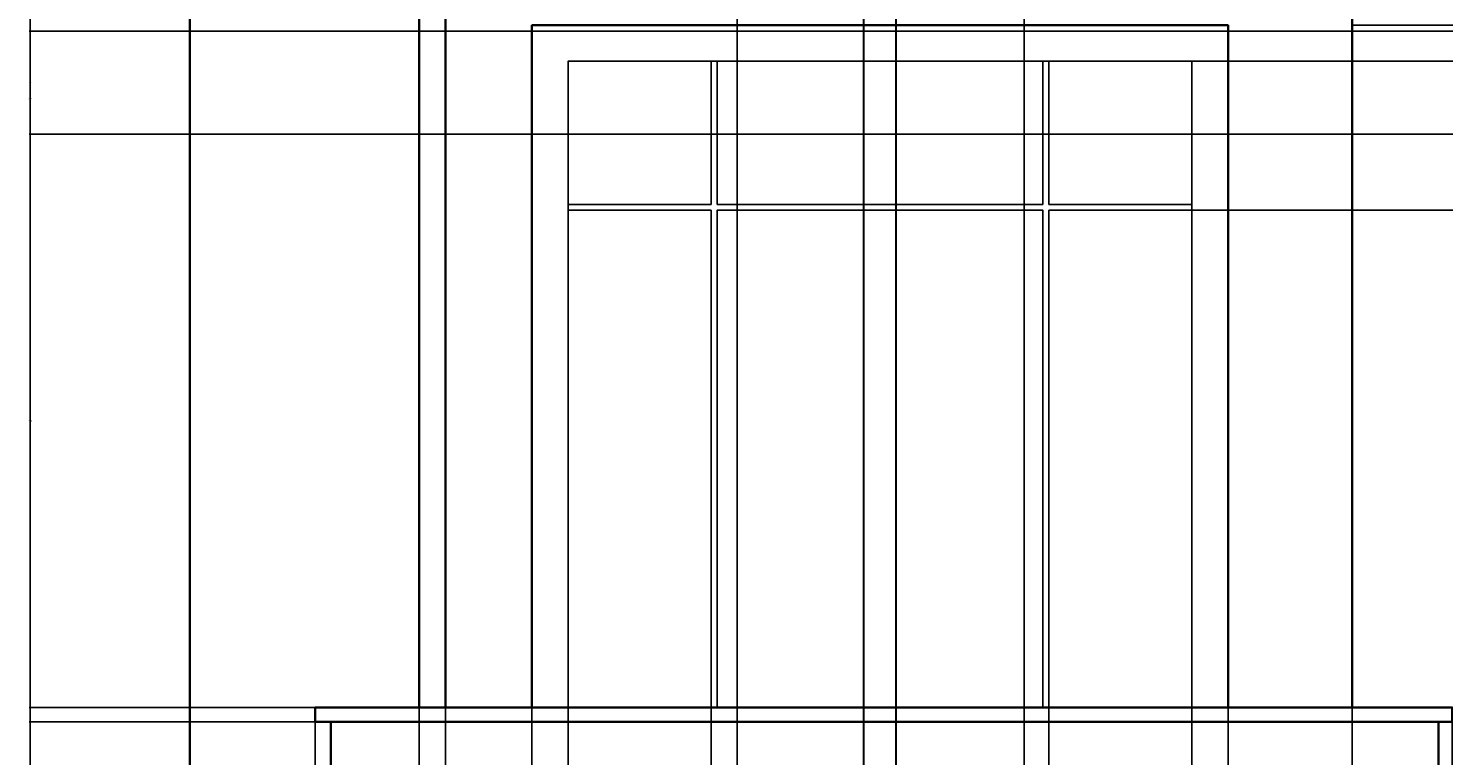
# Model space of a CAD drawing. Units: feet. Extents: x 4092 to 5585, y 725 to 1390.
# Tile 4 of 7: x 4921 to 5204, y 1001 to 1146. Entities that reach past the tile are written whole.
import ezdxf

# ---------------------------------------------------------------- set-up
doc = ezdxf.new("R2010")
doc.units = ezdxf.units.FT
for name, color, linetype, lineweight in [('A-ANNO-DIMS', 2, 'Continuous', 18), ('A-ELEV', 7, 'Continuous', 35), ('A-GLAZ', 4, 'Continuous', 25)]:
    doc.layers.add(name, color=color, linetype=linetype, lineweight=lineweight)
doc.styles.get("Standard").update_dxf_attribs({"font": 'arial.ttf'})
doc.dimstyles.get("Standard").update_dxf_attribs({"dimtxt": 0.18, "dimasz": 0.18, "dimexe": 0.18, "dimexo": 0.0625, "dimgap": 0.09, "dimtad": 0, "dimtih": 1, "dimtoh": 1, "dimdec": 1, "dimzin": 0, "dimdsep": 46, "dimlunit": 3, "dimtxsty": 'Standard', "dimcen": 0.09, "dimadec": 0, "dimazin": 0, "dimtfac": 1, "dimtdec": 1, "dimtofl": 0, "dimtmove": 0, "dimatfit": 3, "dimfxl": 1, "dimtolj": 1, "dimtzin": 0, "dimarcsym": 0})

# ---------------------------------------------------------------- blocks, each defined once
blk = doc.blocks.new('*D18')
at = {"layer": 'A-ANNO-DIMS', "color": 0, "lineweight": -2, "transparency": 16777216}
for p, q in [((4978.29, 1010.79), (4921.27, 1010.79)), ((4921.45, 1010.61), (4921.45, 981.18)), ((4921.45, 951.38), (4921.45, 980.81)), ((5021.54, 951.2), (4921.27, 951.2))]:
    blk.add_line(p, q, dxfattribs=at)
at = {"layer": 'A-ANNO-DIMS', "color": 0, "transparency": 16777216}
for points in [[(4921.42, 1010.61), (4921.48, 1010.61), (4921.45, 1010.79)], [(4921.42, 951.38), (4921.48, 951.38), (4921.45, 951.2)]]:
    blk.add_solid(points, dxfattribs=at)
at = {"layer": 'Defpoints', "color": 0, "transparency": 16777216}
for p in [(4921.45, 1010.79), (4978.36, 1010.79), (5021.61, 951.2)]:
    blk.add_point(p, dxfattribs=at)
at = {"layer": 'A-ANNO-DIMS', "color": 0, "transparency": 16777216, "insert": (4921.45, 981), "char_height": 0.18, "attachment_point": 5}
blk.add_mtext('\\A1;59.59', dxfattribs=at)
blk = doc.blocks.new('*D19')
at = {"layer": 'A-ANNO-DIMS', "color": 0, "lineweight": -2, "transparency": 16777216}
for p, q in [((4953.23, 1253.95), (4921.27, 1253.95)), ((4921.45, 1253.77), (4921.45, 1132.55)), ((4921.45, 1010.97), (4921.45, 1132.19)), ((4978.29, 1010.79), (4921.27, 1010.79))]:
    blk.add_line(p, q, dxfattribs=at)
at = {"layer": 'A-ANNO-DIMS', "color": 0, "transparency": 16777216}
for points in [[(4921.42, 1253.77), (4921.48, 1253.77), (4921.45, 1253.95)], [(4921.42, 1010.97), (4921.48, 1010.97), (4921.45, 1010.79)]]:
    blk.add_solid(points, dxfattribs=at)
at = {"layer": 'Defpoints', "color": 0, "transparency": 16777216}
for p in [(4921.45, 1253.95), (4953.29, 1253.95), (4978.36, 1010.79)]:
    blk.add_point(p, dxfattribs=at)
at = {"layer": 'A-ANNO-DIMS', "color": 0, "transparency": 16777216, "insert": (4921.45, 1132.37), "char_height": 0.18, "attachment_point": 5}
blk.add_mtext('\\A1;243.16', dxfattribs=at)
blk = doc.blocks.new('*D39')
at = {"layer": 'A-ANNO-DIMS', "color": 0, "lineweight": -2, "transparency": 16777216}
for p, q in [((5087.84, 808.72), (5087.84, 1389.85)), ((5088.02, 1389.67), (5090.69, 1389.67)), ((5094.12, 1389.67), (5091.45, 1389.67)), ((5094.3, 808.72), (5094.3, 1389.85))]:
    blk.add_line(p, q, dxfattribs=at)
at = {"layer": 'A-ANNO-DIMS', "color": 0, "transparency": 16777216}
for points in [[(5088.02, 1389.7), (5088.02, 1389.64), (5087.84, 1389.67)], [(5094.12, 1389.7), (5094.12, 1389.64), (5094.3, 1389.67)]]:
    blk.add_solid(points, dxfattribs=at)
at = {"layer": 'Defpoints', "color": 0, "transparency": 16777216}
for p in [(5094.3, 1389.67), (5087.84, 808.65), (5094.3, 808.65)]:
    blk.add_point(p, dxfattribs=at)
at = {"layer": 'A-ANNO-DIMS', "color": 0, "transparency": 16777216, "insert": (5091.07, 1389.67), "char_height": 0.18, "attachment_point": 5}
blk.add_mtext('\\A1;6.461', dxfattribs=at)
blk = doc.blocks.new('*D40')
at = {"layer": 'A-ANNO-DIMS', "color": 0, "lineweight": -2, "transparency": 16777216}
for p, q in [((5062.58, 907.22), (5062.58, 1389.85)), ((5062.76, 1389.67), (5074.7, 1389.67)), ((5087.57, 1389.67), (5075.63, 1389.67)), ((5087.75, 907.22), (5087.75, 1389.85))]:
    blk.add_line(p, q, dxfattribs=at)
at = {"layer": 'A-ANNO-DIMS', "color": 0, "transparency": 16777216}
for points in [[(5062.76, 1389.7), (5062.76, 1389.64), (5062.58, 1389.67)], [(5087.57, 1389.7), (5087.57, 1389.64), (5087.75, 1389.67)]]:
    blk.add_solid(points, dxfattribs=at)
at = {"layer": 'Defpoints', "color": 0, "transparency": 16777216}
for p in [(5087.75, 1389.67), (5062.58, 907.16), (5087.75, 907.16)]:
    blk.add_point(p, dxfattribs=at)
at = {"layer": 'A-ANNO-DIMS', "color": 0, "transparency": 16777216, "insert": (5075.16, 1389.67), "char_height": 0.18, "attachment_point": 5}
blk.add_mtext('\\A1;25.164', dxfattribs=at)
blk = doc.blocks.new('*D41')
at = {"layer": 'A-ANNO-DIMS', "color": 0, "lineweight": -2, "transparency": 16777216}
for p, q in [((5087.75, 907.22), (5087.75, 1389.85)), ((5087.93, 1389.67), (5090.59, 1389.67)), ((5094.04, 1389.67), (5091.38, 1389.67)), ((5094.22, 907.22), (5094.22, 1389.85))]:
    blk.add_line(p, q, dxfattribs=at)
at = {"layer": 'A-ANNO-DIMS', "color": 0, "transparency": 16777216}
for points in [[(5087.93, 1389.7), (5087.93, 1389.64), (5087.75, 1389.67)], [(5094.04, 1389.7), (5094.04, 1389.64), (5094.22, 1389.67)]]:
    blk.add_solid(points, dxfattribs=at)
at = {"layer": 'Defpoints', "color": 0, "transparency": 16777216}
for p in [(5094.22, 1389.67), (5087.75, 907.16), (5094.22, 907.16)]:
    blk.add_point(p, dxfattribs=at)
at = {"layer": 'A-ANNO-DIMS', "color": 0, "transparency": 16777216, "insert": (5090.98, 1389.67), "char_height": 0.18, "attachment_point": 5}
blk.add_mtext('\\A1;6.474', dxfattribs=at)
blk = doc.blocks.new('*D42')
at = {"layer": 'A-ANNO-DIMS', "color": 0, "lineweight": -2, "transparency": 16777216}
for p, q in [((5094.22, 907.22), (5094.22, 1389.85)), ((5094.4, 1389.67), (5106.69, 1389.67)), ((5119.64, 1389.67), (5107.34, 1389.67)), ((5119.82, 907.22), (5119.82, 1389.85))]:
    blk.add_line(p, q, dxfattribs=at)
at = {"layer": 'A-ANNO-DIMS', "color": 0, "transparency": 16777216}
for points in [[(5094.4, 1389.7), (5094.4, 1389.64), (5094.22, 1389.67)], [(5119.64, 1389.7), (5119.64, 1389.64), (5119.82, 1389.67)]]:
    blk.add_solid(points, dxfattribs=at)
at = {"layer": 'Defpoints', "color": 0, "transparency": 16777216}
for p in [(5119.82, 1389.67), (5094.22, 907.16), (5119.82, 907.16)]:
    blk.add_point(p, dxfattribs=at)
at = {"layer": 'A-ANNO-DIMS', "color": 0, "transparency": 16777216, "insert": (5107.02, 1389.67), "char_height": 0.18, "attachment_point": 5}
blk.add_mtext('\\A1;25.6', dxfattribs=at)
blk = doc.blocks.new('*D46')
at = {"layer": 'A-ANNO-DIMS', "color": 0, "lineweight": -2, "transparency": 16777216}
for p, q in [((4978.29, 1007.95), (4921.27, 1007.95)), ((4921.45, 1007.77), (4921.45, 986.89)), ((4921.45, 965.66), (4921.45, 986.53)), ((4981.38, 965.48), (4921.27, 965.48))]:
    blk.add_line(p, q, dxfattribs=at)
at = {"layer": 'A-ANNO-DIMS', "color": 0, "transparency": 16777216}
for points in [[(4921.42, 1007.77), (4921.48, 1007.77), (4921.45, 1007.95)], [(4921.42, 965.66), (4921.48, 965.66), (4921.45, 965.48)]]:
    blk.add_solid(points, dxfattribs=at)
at = {"layer": 'Defpoints', "color": 0, "transparency": 16777216}
for p in [(4921.45, 1007.95), (4978.36, 1007.95), (4981.44, 965.48)]:
    blk.add_point(p, dxfattribs=at)
at = {"layer": 'A-ANNO-DIMS', "color": 0, "transparency": 16777216, "insert": (4921.45, 986.71), "char_height": 0.18, "attachment_point": 5}
blk.add_mtext('\\A1;42.47', dxfattribs=at)
blk = doc.blocks.new('*D47')
at = {"layer": 'A-ANNO-DIMS', "color": 0, "lineweight": -2, "transparency": 16777216}
for p, q in [((4978.36, 1010.73), (4978.36, 725.07)), ((4999.11, 1010.73), (4999.11, 725.07)), ((4978.54, 725.25), (4988.34, 725.25)), ((4998.93, 725.25), (4989.13, 725.25))]:
    blk.add_line(p, q, dxfattribs=at)
at = {"layer": 'A-ANNO-DIMS', "color": 0, "transparency": 16777216}
for points in [[(4978.54, 725.28), (4978.54, 725.22), (4978.36, 725.25)], [(4998.93, 725.28), (4998.93, 725.22), (4999.11, 725.25)]]:
    blk.add_solid(points, dxfattribs=at)
at = {"layer": 'Defpoints', "color": 0, "transparency": 16777216}
for p in [(4978.36, 1010.79), (4999.11, 1010.79), (4999.11, 725.25)]:
    blk.add_point(p, dxfattribs=at)
at = {"layer": 'A-ANNO-DIMS', "color": 0, "transparency": 16777216, "insert": (4988.74, 725.25), "char_height": 0.18, "attachment_point": 5}
blk.add_mtext('\\A1;20.76', dxfattribs=at)
blk = doc.blocks.new('*D48')
at = {"layer": 'A-ANNO-DIMS', "color": 0, "lineweight": -2, "transparency": 16777216}
for p, q in [((4999.11, 1010.73), (4999.11, 725.07)), ((5004.32, 1010.73), (5004.32, 725.07)), ((4999.29, 725.25), (5001.32, 725.25)), ((5004.14, 725.25), (5002.11, 725.25))]:
    blk.add_line(p, q, dxfattribs=at)
at = {"layer": 'A-ANNO-DIMS', "color": 0, "transparency": 16777216}
for points in [[(4999.29, 725.28), (4999.29, 725.22), (4999.11, 725.25)], [(5004.14, 725.28), (5004.14, 725.22), (5004.32, 725.25)]]:
    blk.add_solid(points, dxfattribs=at)
at = {"layer": 'Defpoints', "color": 0, "transparency": 16777216}
for p in [(4999.11, 1010.79), (5004.32, 1010.79), (5004.32, 725.25)]:
    blk.add_point(p, dxfattribs=at)
at = {"layer": 'A-ANNO-DIMS', "color": 0, "transparency": 16777216, "insert": (5001.72, 725.25), "char_height": 0.18, "attachment_point": 5}
blk.add_mtext('\\A1;5.203', dxfattribs=at)
blk = doc.blocks.new('*D49')
at = {"layer": 'A-ANNO-DIMS', "color": 0, "lineweight": -2, "transparency": 16777216}
for p, q in [((5004.32, 1010.73), (5004.32, 725.07)), ((5021.61, 1010.73), (5021.61, 725.07)), ((5004.5, 725.25), (5012.58, 725.25)), ((5021.43, 725.25), (5013.35, 725.25))]:
    blk.add_line(p, q, dxfattribs=at)
at = {"layer": 'A-ANNO-DIMS', "color": 0, "transparency": 16777216}
for points in [[(5004.5, 725.28), (5004.5, 725.22), (5004.32, 725.25)], [(5021.43, 725.28), (5021.43, 725.22), (5021.61, 725.25)]]:
    blk.add_solid(points, dxfattribs=at)
at = {"layer": 'Defpoints', "color": 0, "transparency": 16777216}
for p in [(5004.32, 1010.79), (5021.61, 1010.79), (5021.61, 725.25)]:
    blk.add_point(p, dxfattribs=at)
at = {"layer": 'A-ANNO-DIMS', "color": 0, "transparency": 16777216, "insert": (5012.96, 725.25), "char_height": 0.18, "attachment_point": 5}
blk.add_mtext('\\A1;17.29', dxfattribs=at)
blk = doc.blocks.new('*D50')
at = {"layer": 'A-ANNO-DIMS', "color": 0, "lineweight": -2, "transparency": 16777216}
for p, q in [((5021.61, 1010.73), (5021.61, 725.07)), ((5028.8, 1010.73), (5028.8, 725.07)), ((5021.79, 725.25), (5024.81, 725.25)), ((5028.62, 725.25), (5025.6, 725.25))]:
    blk.add_line(p, q, dxfattribs=at)
at = {"layer": 'A-ANNO-DIMS', "color": 0, "transparency": 16777216}
for points in [[(5021.79, 725.28), (5021.79, 725.22), (5021.61, 725.25)], [(5028.62, 725.28), (5028.62, 725.22), (5028.8, 725.25)]]:
    blk.add_solid(points, dxfattribs=at)
at = {"layer": 'Defpoints', "color": 0, "transparency": 16777216}
for p in [(5021.61, 1010.79), (5028.8, 1010.79), (5028.8, 725.25)]:
    blk.add_point(p, dxfattribs=at)
at = {"layer": 'A-ANNO-DIMS', "color": 0, "transparency": 16777216, "insert": (5025.2, 725.25), "char_height": 0.18, "attachment_point": 5}
blk.add_mtext('\\A1;7.194', dxfattribs=at)
blk = doc.blocks.new('*D51')
at = {"layer": 'A-ANNO-DIMS', "color": 0, "lineweight": -2, "transparency": 16777216}
for p, q in [((5028.8, 1010.73), (5028.8, 725.07)), ((5057.39, 1010.73), (5057.39, 725.07)), ((5028.98, 725.25), (5042.7, 725.25)), ((5057.21, 725.25), (5043.49, 725.25))]:
    blk.add_line(p, q, dxfattribs=at)
at = {"layer": 'A-ANNO-DIMS', "color": 0, "transparency": 16777216}
for points in [[(5028.98, 725.28), (5028.98, 725.22), (5028.8, 725.25)], [(5057.21, 725.28), (5057.21, 725.22), (5057.39, 725.25)]]:
    blk.add_solid(points, dxfattribs=at)
at = {"layer": 'Defpoints', "color": 0, "transparency": 16777216}
for p in [(5028.8, 1010.79), (5057.39, 1010.79), (5057.39, 725.25)]:
    blk.add_point(p, dxfattribs=at)
at = {"layer": 'A-ANNO-DIMS', "color": 0, "transparency": 16777216, "insert": (5043.1, 725.25), "char_height": 0.18, "attachment_point": 5}
blk.add_mtext('\\A1;28.59', dxfattribs=at)
blk = doc.blocks.new('*D52')
at = {"layer": 'A-ANNO-DIMS', "color": 0, "lineweight": -2, "transparency": 16777216}
for p, q in [((5057.39, 1010.73), (5057.39, 725.07)), ((5124.75, 1010.73), (5124.75, 725.07)), ((5057.57, 725.25), (5090.68, 725.25)), ((5124.57, 725.25), (5091.46, 725.25))]:
    blk.add_line(p, q, dxfattribs=at)
at = {"layer": 'A-ANNO-DIMS', "color": 0, "transparency": 16777216}
for points in [[(5057.57, 725.28), (5057.57, 725.22), (5057.39, 725.25)], [(5124.57, 725.28), (5124.57, 725.22), (5124.75, 725.25)]]:
    blk.add_solid(points, dxfattribs=at)
at = {"layer": 'Defpoints', "color": 0, "transparency": 16777216}
for p in [(5057.39, 1010.79), (5124.75, 1010.79), (5124.75, 725.25)]:
    blk.add_point(p, dxfattribs=at)
at = {"layer": 'A-ANNO-DIMS', "color": 0, "transparency": 16777216, "insert": (5091.07, 725.25), "char_height": 0.18, "attachment_point": 5}
blk.add_mtext('\\A1;67.36', dxfattribs=at)
blk = doc.blocks.new('*D53')
at = {"layer": 'A-ANNO-DIMS', "color": 0, "lineweight": -2, "transparency": 16777216}
for p, q in [((5124.75, 1010.73), (5124.75, 725.07)), ((5153.34, 1010.73), (5153.34, 725.07)), ((5124.93, 725.25), (5138.65, 725.25)), ((5153.16, 725.25), (5139.44, 725.25))]:
    blk.add_line(p, q, dxfattribs=at)
at = {"layer": 'A-ANNO-DIMS', "color": 0, "transparency": 16777216}
for points in [[(5124.93, 725.28), (5124.93, 725.22), (5124.75, 725.25)], [(5153.16, 725.28), (5153.16, 725.22), (5153.34, 725.25)]]:
    blk.add_solid(points, dxfattribs=at)
at = {"layer": 'Defpoints', "color": 0, "transparency": 16777216}
for p in [(5124.75, 1010.79), (5153.34, 1010.79), (5153.34, 725.25)]:
    blk.add_point(p, dxfattribs=at)
at = {"layer": 'A-ANNO-DIMS', "color": 0, "transparency": 16777216, "insert": (5139.04, 725.25), "char_height": 0.18, "attachment_point": 5}
blk.add_mtext('\\A1;28.59', dxfattribs=at)
blk = doc.blocks.new('*D54')
at = {"layer": 'A-ANNO-DIMS', "color": 0, "lineweight": -2, "transparency": 16777216}
for p, q in [((5153.34, 1010.73), (5153.34, 725.07)), ((5160.53, 1010.73), (5160.53, 725.07)), ((5153.52, 725.25), (5156.54, 725.25)), ((5160.35, 725.25), (5157.33, 725.25))]:
    blk.add_line(p, q, dxfattribs=at)
at = {"layer": 'A-ANNO-DIMS', "color": 0, "transparency": 16777216}
for points in [[(5153.52, 725.28), (5153.52, 725.22), (5153.34, 725.25)], [(5160.35, 725.28), (5160.35, 725.22), (5160.53, 725.25)]]:
    blk.add_solid(points, dxfattribs=at)
at = {"layer": 'Defpoints', "color": 0, "transparency": 16777216}
for p in [(5153.34, 1010.79), (5160.53, 1010.79), (5160.53, 725.25)]:
    blk.add_point(p, dxfattribs=at)
at = {"layer": 'A-ANNO-DIMS', "color": 0, "transparency": 16777216, "insert": (5156.94, 725.25), "char_height": 0.18, "attachment_point": 5}
blk.add_mtext('\\A1;7.194', dxfattribs=at)
blk = doc.blocks.new('*D55')
at = {"layer": 'A-ANNO-DIMS', "color": 0, "lineweight": -2, "transparency": 16777216}
for p, q in [((5160.53, 1010.73), (5160.53, 725.07)), ((5185.33, 1010.73), (5185.33, 725.07)), ((5160.71, 725.25), (5172.47, 725.25)), ((5185.15, 725.25), (5173.4, 725.25))]:
    blk.add_line(p, q, dxfattribs=at)
at = {"layer": 'A-ANNO-DIMS', "color": 0, "transparency": 16777216}
for points in [[(5160.71, 725.28), (5160.71, 725.22), (5160.53, 725.25)], [(5185.15, 725.28), (5185.15, 725.22), (5185.33, 725.25)]]:
    blk.add_solid(points, dxfattribs=at)
at = {"layer": 'Defpoints', "color": 0, "transparency": 16777216}
for p in [(5160.53, 1010.79), (5185.33, 1010.79), (5185.33, 725.25)]:
    blk.add_point(p, dxfattribs=at)
at = {"layer": 'A-ANNO-DIMS', "color": 0, "transparency": 16777216, "insert": (5172.93, 725.25), "char_height": 0.18, "attachment_point": 5}
blk.add_mtext('\\A1;24.796', dxfattribs=at)
blk = doc.blocks.new('*D56')
at = {"layer": 'A-ANNO-DIMS', "color": 0, "lineweight": -2, "transparency": 16777216}
for p, q in [((5185.33, 1010.73), (5185.33, 725.07)), ((5205.28, 1010.73), (5205.28, 725.07)), ((5185.51, 725.25), (5194.85, 725.25)), ((5205.1, 725.25), (5195.76, 725.25))]:
    blk.add_line(p, q, dxfattribs=at)
at = {"layer": 'A-ANNO-DIMS', "color": 0, "transparency": 16777216}
for points in [[(5185.51, 725.28), (5185.51, 725.22), (5185.33, 725.25)], [(5205.1, 725.28), (5205.1, 725.22), (5205.28, 725.25)]]:
    blk.add_solid(points, dxfattribs=at)
at = {"layer": 'Defpoints', "color": 0, "transparency": 16777216}
for p in [(5185.33, 1010.79), (5205.28, 1010.79), (5205.28, 725.25)]:
    blk.add_point(p, dxfattribs=at)
at = {"layer": 'A-ANNO-DIMS', "color": 0, "transparency": 16777216, "insert": (5195.3, 725.25), "char_height": 0.18, "attachment_point": 5}
blk.add_mtext('\\A1;19.947', dxfattribs=at)
blk = doc.blocks.new('*D57')
at = {"layer": 'A-ANNO-DIMS', "color": 0, "lineweight": -2, "transparency": 16777216}
for p, q in [((5153.4, 1110.12), (5584.71, 1110.12)), ((5584.53, 1109.94), (5584.53, 1060.64)), ((5584.53, 1010.97), (5584.53, 1060.27)), ((5185.39, 1010.79), (5584.71, 1010.79))]:
    blk.add_line(p, q, dxfattribs=at)
at = {"layer": 'A-ANNO-DIMS', "color": 0, "transparency": 16777216}
for points in [[(5584.5, 1109.94), (5584.56, 1109.94), (5584.53, 1110.12)], [(5584.5, 1010.97), (5584.56, 1010.97), (5584.53, 1010.79)]]:
    blk.add_solid(points, dxfattribs=at)
at = {"layer": 'Defpoints', "color": 0, "transparency": 16777216}
for p in [(5153.34, 1110.12), (5584.53, 1110.12), (5185.33, 1010.79)]:
    blk.add_point(p, dxfattribs=at)
at = {"layer": 'A-ANNO-DIMS', "color": 0, "transparency": 16777216, "insert": (5584.53, 1060.45), "char_height": 0.18, "attachment_point": 5}
blk.add_mtext('\\A1;99.33', dxfattribs=at)
blk = doc.blocks.new('*D58')
at = {"layer": 'A-ANNO-DIMS', "color": 0, "lineweight": -2, "transparency": 16777216}
for p, q in [((5153.4, 1139.88), (5584.71, 1139.88)), ((5584.53, 1139.7), (5584.53, 1125.18)), ((5584.53, 1110.3), (5584.53, 1124.82)), ((5153.4, 1110.12), (5584.71, 1110.12))]:
    blk.add_line(p, q, dxfattribs=at)
at = {"layer": 'A-ANNO-DIMS', "color": 0, "transparency": 16777216}
for points in [[(5584.5, 1139.7), (5584.56, 1139.7), (5584.53, 1139.88)], [(5584.5, 1110.3), (5584.56, 1110.3), (5584.53, 1110.12)]]:
    blk.add_solid(points, dxfattribs=at)
at = {"layer": 'Defpoints', "color": 0, "transparency": 16777216}
for p in [(5153.34, 1139.88), (5584.53, 1139.88), (5153.34, 1110.12)]:
    blk.add_point(p, dxfattribs=at)
at = {"layer": 'A-ANNO-DIMS', "color": 0, "transparency": 16777216, "insert": (5584.53, 1125), "char_height": 0.18, "attachment_point": 5}
blk.add_mtext('\\A1;29.76', dxfattribs=at)
blk = doc.blocks.new('*D59')
at = {"layer": 'A-ANNO-DIMS', "color": 0, "lineweight": -2, "transparency": 16777216}
for p, q in [((5185.39, 1147.07), (5584.71, 1147.07)), ((5584.53, 1146.89), (5584.53, 1143.66)), ((5584.53, 1140.06), (5584.53, 1143.3)), ((5153.4, 1139.88), (5584.71, 1139.88))]:
    blk.add_line(p, q, dxfattribs=at)
at = {"layer": 'A-ANNO-DIMS', "color": 0, "transparency": 16777216}
for points in [[(5584.5, 1146.89), (5584.56, 1146.89), (5584.53, 1147.07)], [(5584.5, 1140.06), (5584.56, 1140.06), (5584.53, 1139.88)]]:
    blk.add_solid(points, dxfattribs=at)
at = {"layer": 'Defpoints', "color": 0, "transparency": 16777216}
for p in [(5185.33, 1147.07), (5584.53, 1147.07), (5153.34, 1139.88)]:
    blk.add_point(p, dxfattribs=at)
at = {"layer": 'A-ANNO-DIMS', "color": 0, "transparency": 16777216, "insert": (5584.53, 1143.48), "char_height": 0.18, "attachment_point": 5}
blk.add_mtext('\\A1;7.194', dxfattribs=at)
blk = doc.blocks.new('*D78')
at = {"layer": 'A-ANNO-DIMS', "color": 0, "lineweight": -2, "transparency": 16777216}
for p, q in [((5392.49, 1007.95), (4921.27, 1007.95)), ((4921.45, 1007.77), (4921.45, 986.89)), ((4921.45, 965.66), (4921.45, 986.53)), ((5392.49, 965.48), (4921.27, 965.48))]:
    blk.add_line(p, q, dxfattribs=at)
at = {"layer": 'A-ANNO-DIMS', "color": 0, "transparency": 16777216}
for points in [[(4921.42, 1007.77), (4921.48, 1007.77), (4921.45, 1007.95)], [(4921.42, 965.66), (4921.48, 965.66), (4921.45, 965.48)]]:
    blk.add_solid(points, dxfattribs=at)
at = {"layer": 'Defpoints', "color": 0, "transparency": 16777216}
for p in [(4921.45, 1007.95), (5392.55, 1007.95), (5392.55, 965.48)]:
    blk.add_point(p, dxfattribs=at)
at = {"layer": 'A-ANNO-DIMS', "color": 0, "transparency": 16777216, "insert": (4921.45, 986.71), "char_height": 0.18, "attachment_point": 5}
blk.add_mtext('\\A1;42.47', dxfattribs=at)
blk = doc.blocks.new('*D79')
at = {"layer": 'A-ANNO-DIMS', "color": 0, "lineweight": -2, "transparency": 16777216}
for p, q in [((5392.49, 1125.34), (4921.27, 1125.34)), ((4921.45, 1125.16), (4921.45, 1068.25)), ((4921.45, 1010.97), (4921.45, 1067.88)), ((5392.49, 1010.79), (4921.27, 1010.79))]:
    blk.add_line(p, q, dxfattribs=at)
at = {"layer": 'A-ANNO-DIMS', "color": 0, "transparency": 16777216}
for points in [[(4921.42, 1125.16), (4921.48, 1125.16), (4921.45, 1125.34)], [(4921.42, 1010.97), (4921.48, 1010.97), (4921.45, 1010.79)]]:
    blk.add_solid(points, dxfattribs=at)
at = {"layer": 'Defpoints', "color": 0, "transparency": 16777216}
for p in [(4921.45, 1125.34), (5392.55, 1125.34), (5392.55, 1010.79)]:
    blk.add_point(p, dxfattribs=at)
at = {"layer": 'A-ANNO-DIMS', "color": 0, "transparency": 16777216, "insert": (4921.45, 1068.07), "char_height": 0.18, "attachment_point": 5}
blk.add_mtext('\\A1;114.55', dxfattribs=at)
blk = doc.blocks.new('*D80')
at = {"layer": 'A-ANNO-DIMS', "color": 0, "lineweight": -2, "transparency": 16777216}
for p, q in [((5392.49, 1145.86), (4921.27, 1145.86)), ((4921.45, 1145.68), (4921.45, 1135.78)), ((4921.45, 1125.52), (4921.45, 1135.42)), ((5392.49, 1125.34), (4921.27, 1125.34))]:
    blk.add_line(p, q, dxfattribs=at)
at = {"layer": 'A-ANNO-DIMS', "color": 0, "transparency": 16777216}
for points in [[(4921.42, 1145.68), (4921.48, 1145.68), (4921.45, 1145.86)], [(4921.42, 1125.52), (4921.48, 1125.52), (4921.45, 1125.34)]]:
    blk.add_solid(points, dxfattribs=at)
at = {"layer": 'Defpoints', "color": 0, "transparency": 16777216}
for p in [(4921.45, 1145.86), (5392.55, 1145.86), (5392.55, 1125.34)]:
    blk.add_point(p, dxfattribs=at)
at = {"layer": 'A-ANNO-DIMS', "color": 0, "transparency": 16777216, "insert": (4921.45, 1135.6), "char_height": 0.18, "attachment_point": 5}
blk.add_mtext('\\A1;20.52', dxfattribs=at)
blk = doc.blocks.new('*D81')
at = {"layer": 'A-ANNO-DIMS', "color": 0, "lineweight": -2, "transparency": 16777216}
for p, q in [((5392.49, 1171.51), (4921.27, 1171.51)), ((4921.45, 1171.33), (4921.45, 1158.87)), ((4921.45, 1146.04), (4921.45, 1158.5)), ((5392.49, 1145.86), (4921.27, 1145.86))]:
    blk.add_line(p, q, dxfattribs=at)
at = {"layer": 'A-ANNO-DIMS', "color": 0, "transparency": 16777216}
for points in [[(4921.42, 1171.33), (4921.48, 1171.33), (4921.45, 1171.51)], [(4921.42, 1146.04), (4921.48, 1146.04), (4921.45, 1145.86)]]:
    blk.add_solid(points, dxfattribs=at)
at = {"layer": 'Defpoints', "color": 0, "transparency": 16777216}
for p in [(4921.45, 1171.51), (5392.55, 1171.51), (5392.55, 1145.86)]:
    blk.add_point(p, dxfattribs=at)
at = {"layer": 'A-ANNO-DIMS', "color": 0, "transparency": 16777216, "insert": (4921.45, 1158.69), "char_height": 0.18, "attachment_point": 5}
blk.add_mtext('\\A1;25.65', dxfattribs=at)

msp = doc.modelspace()

# ---------------------------------------------------------------- linework, layer by layer
at = {"layer": 'A-ELEV'}
for p, q in [((4953.293, 755.9488), (4953.293, 1253.9488)), ((5021.6062, 1010.7906), (5160.5329, 1010.7906))]:
    msp.add_line(p, q, dxfattribs=at)
for points in [[(4953.293, 755.9488), (5231.15, 755.9488), (5231.15, 1253.9488), (4953.293, 1253.9488)], [(4978.356, 1007.9488), (5205.2757, 1007.9488), (5205.2757, 1010.7906), (4978.356, 1010.7906)], [(4981.4448, 1007.9488), (5202.5428, 1007.9488), (5202.5428, 965.4789), (4981.4448, 965.4789)]]:
    msp.add_lwpolyline(points, close=True, dxfattribs=at)
for points in [[(5185.3285, 1010.7906), (5185.3285, 1208.1273), (4999.1145, 1208.1273), (4999.1145, 1010.7906)], [(5185.3285, 1202.9247), (5004.3171, 1202.9247), (5004.3171, 1010.7906)], [(5021.6062, 1010.7906), (5021.6062, 1147.0743), (5160.5329, 1147.0743), (5160.5329, 1010.7906)]]:
    msp.add_lwpolyline(points, dxfattribs=at)
at = {"layer": 'A-GLAZ'}
for p, q in [((5057.3906, 1111.2899), (5057.3906, 1139.8803)), ((5058.5615, 1111.2899), (5058.5615, 1139.8803)), ((5123.5775, 1111.2899), (5123.5775, 1139.8803)), ((5124.7484, 1111.2899), (5124.7484, 1139.8803)), ((5057.3906, 1111.2899), (5028.8002, 1111.2899)), ((5124.7484, 1111.2899), (5153.3388, 1111.2899)), ((5057.3906, 1110.119), (5028.8002, 1110.119)), ((5124.7484, 1110.119), (5153.3388, 1110.119))]:
    msp.add_line(p, q, dxfattribs=at)
for points in [[(5028.8002, 1010.7906), (5028.8002, 1139.8803), (5153.3388, 1139.8803), (5153.3388, 1010.7906)], [(5058.5615, 1111.2899), (5123.5775, 1111.2899)], [(5057.3906, 1010.7906), (5057.3906, 1110.119)], [(5058.5615, 1010.7906), (5058.5615, 1110.119), (5123.5775, 1110.119), (5123.5775, 1010.7906)], [(5124.7484, 1110.119), (5124.7484, 1010.7906)]]:
    msp.add_lwpolyline(points, dxfattribs=at)

# ---------------------------------------------------------------- dimensions: what is measured, and where the dimension line sits
at = {"layer": 'A-ANNO-DIMS'}
for base, p1, p2, override, picture, middle in [((5087.7457, 1389.6731), (5062.5819, 907.159), (5087.7457, 907.159), {"dimdec": 3, "dimlfac": 1, "dimrnd": 0, "dimzin": 0, "dimdsep": 46, "dimlunit": 2}, '*D40', (5075.1638, 1389.6731)), ((5094.2195, 1389.6731), (5087.7457, 907.159), (5094.2195, 907.159), {"dimdec": 3, "dimlfac": 1, "dimrnd": 0, "dimzin": 0, "dimdsep": 46, "dimlunit": 2}, '*D41', (5090.9826, 1389.6731)), ((5094.3002, 1389.6731), (5087.8389, 808.6527), (5094.3002, 808.6527), {"dimdec": 3, "dimlfac": 1, "dimrnd": 0, "dimzin": 0, "dimdsep": 46, "dimlunit": 2}, '*D39', (5091.0695, 1389.6731)), ((5119.8191, 1389.6731), (5094.2195, 907.159), (5119.8191, 907.159), {"dimdec": 1, "dimlfac": 1, "dimrnd": 0, "dimzin": 0, "dimdsep": 46, "dimlunit": 2}, '*D42', (5107.0193, 1389.6731)), ((4999.1145, 725.2488), (4978.356, 1010.7906), (4999.1145, 1010.7906), {"dimdec": 2, "dimlfac": 1, "dimrnd": 0, "dimzin": 0, "dimdsep": 46, "dimlunit": 2}, '*D47', (4988.7353, 725.2488)), ((5004.3171, 725.2488), (4999.1145, 1010.7906), (5004.3171, 1010.7906), {"dimdec": 3, "dimlfac": 1, "dimrnd": 0, "dimzin": 0, "dimdsep": 46, "dimlunit": 2}, '*D48', (5001.7158, 725.2488)), ((5021.6062, 725.2488), (5004.3171, 1010.7906), (5021.6062, 1010.7906), {"dimdec": 2, "dimlfac": 1, "dimrnd": 0, "dimzin": 0, "dimdsep": 46, "dimlunit": 2}, '*D49', (5012.9616, 725.2488)), ((5028.8002, 725.2488), (5021.6062, 1010.7906), (5028.8002, 1010.7906), {"dimdec": 3, "dimlfac": 1, "dimrnd": 0, "dimzin": 0, "dimdsep": 46, "dimlunit": 2}, '*D50', (5025.2032, 725.2488)), ((5057.3906, 725.2488), (5028.8002, 1010.7906), (5057.3906, 1010.7906), {"dimdec": 2, "dimlfac": 1, "dimrnd": 0, "dimzin": 0, "dimdsep": 46, "dimlunit": 2}, '*D51', (5043.0954, 725.2488)), ((5124.7484, 725.2488), (5057.3906, 1010.7906), (5124.7484, 1010.7906), {"dimdec": 2, "dimlfac": 1, "dimrnd": 0, "dimzin": 0, "dimdsep": 46, "dimlunit": 2}, '*D52', (5091.0695, 725.2488)), ((5153.3388, 725.2488), (5124.7484, 1010.7906), (5153.3388, 1010.7906), {"dimdec": 2, "dimlfac": 1, "dimrnd": 0, "dimzin": 0, "dimdsep": 46, "dimlunit": 2}, '*D53', (5139.0436, 725.2488)), ((5160.5329, 725.2488), (5153.3388, 1010.7906), (5160.5329, 1010.7906), {"dimdec": 3, "dimlfac": 1, "dimrnd": 0, "dimzin": 0, "dimdsep": 46, "dimlunit": 2}, '*D54', (5156.9359, 725.2488)), ((5185.3285, 725.2488), (5160.5329, 1010.7906), (5185.3285, 1010.7906), {"dimdec": 3, "dimlfac": 1, "dimrnd": 0, "dimzin": 0, "dimdsep": 46, "dimlunit": 2}, '*D55', (5172.9307, 725.2488)), ((5205.2757, 725.2488), (5185.3285, 1010.7906), (5205.2757, 1010.7906), {"dimdec": 3, "dimlfac": 1, "dimrnd": 0, "dimzin": 0, "dimdsep": 46, "dimlunit": 2}, '*D56', (5195.3021, 725.2488))]:
    dim = msp.add_linear_dim(base=base, p1=p1, p2=p2, dimstyle='Standard', override=override, dxfattribs=at)
    dim.commit()
    dim.dimension.update_dxf_attribs({"geometry": picture, "text_midpoint": middle})
for base, p1, p2, override, picture, middle in [((4921.4517, 1253.9488), (4978.356, 1010.7906), (4953.293, 1253.9488), {"dimdec": 2, "dimlfac": 1, "dimrnd": 0, "dimzin": 0, "dimdsep": 46, "dimlunit": 2}, '*D19', (4921.4517, 1132.3697)), ((4921.4517, 1171.511), (5392.5521, 1145.8611), (5392.5521, 1171.511), {"dimdec": 2, "dimlfac": 1, "dimrnd": 0, "dimzin": 0, "dimdsep": 46, "dimlunit": 2}, '*D81', (4921.4517, 1158.6861)), ((5584.5322, 1147.0743), (5153.3388, 1139.8803), (5185.3285, 1147.0743), {"dimdec": 3, "dimlfac": 1, "dimrnd": 0, "dimzin": 0, "dimdsep": 46, "dimlunit": 2}, '*D59', (5584.5322, 1143.4773)), ((4921.4517, 1145.8611), (5392.5521, 1125.3426), (5392.5521, 1145.8611), {"dimdec": 2, "dimlfac": 1, "dimrnd": 0, "dimzin": 0, "dimdsep": 46, "dimlunit": 2}, '*D80', (4921.4517, 1135.6018)), ((5584.5322, 1139.8803), (5153.3388, 1110.119), (5153.3388, 1139.8803), {"dimdec": 2, "dimlfac": 1, "dimrnd": 0, "dimzin": 0, "dimdsep": 46, "dimlunit": 2}, '*D58', (5584.5322, 1124.9996)), ((4921.4517, 1125.3426), (5392.5521, 1010.7906), (5392.5521, 1125.3426), {"dimdec": 2, "dimlfac": 1, "dimrnd": 0, "dimzin": 0, "dimdsep": 46, "dimlunit": 2}, '*D79', (4921.4517, 1068.0666)), ((5584.5322, 1110.119), (5185.3285, 1010.7906), (5153.3388, 1110.119), {"dimdec": 2, "dimlfac": 1, "dimrnd": 0, "dimzin": 0, "dimdsep": 46, "dimlunit": 2}, '*D57', (5584.5322, 1060.4548)), ((4921.4517, 1010.7906), (5021.6062, 951.2024), (4978.356, 1010.7906), {"dimdec": 2, "dimlfac": 1, "dimrnd": 0, "dimzin": 0, "dimdsep": 46, "dimlunit": 2}, '*D18', (4921.4517, 980.9965)), ((4921.4517, 1007.9488), (4981.4448, 965.4789), (4978.356, 1007.9488), {"dimdec": 2, "dimlfac": 1, "dimrnd": 0, "dimzin": 0, "dimdsep": 46, "dimlunit": 2}, '*D46', (4921.4517, 986.7139)), ((4921.4517, 1007.9488), (5392.5521, 965.4789), (5392.5521, 1007.9488), {"dimdec": 2, "dimlfac": 1, "dimrnd": 0, "dimzin": 0, "dimdsep": 46, "dimlunit": 2}, '*D78', (4921.4517, 986.7139))]:
    dim = msp.add_linear_dim(base=base, p1=p1, p2=p2, angle=90, dimstyle='Standard', override=override, dxfattribs=at)
    dim.commit()
    dim.dimension.update_dxf_attribs({"geometry": picture, "text_midpoint": middle})

doc.saveas('drawing.dxf')
